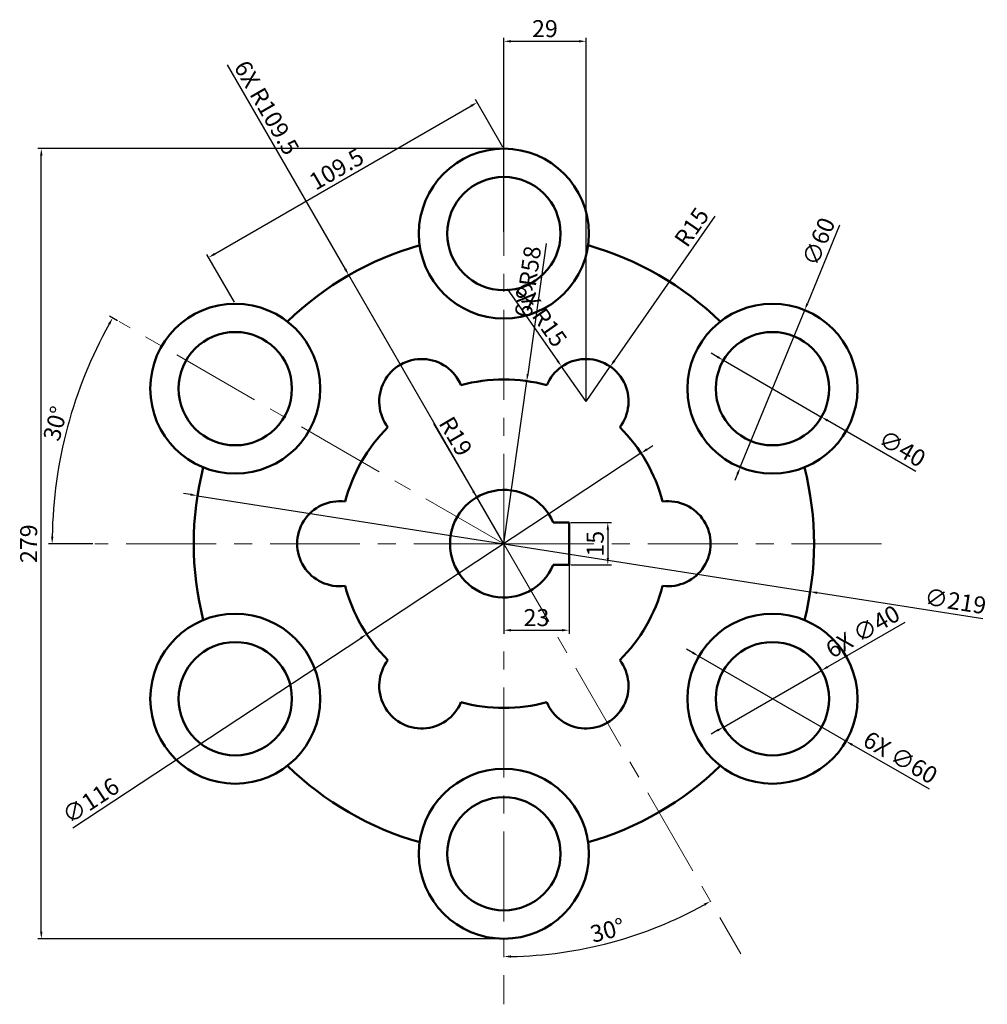
# Model space of a CAD drawing. Units: millimetres. Extents: x 3066 to 3408, y 1460 to 1808.
import ezdxf

# ---------------------------------------------------------------- set-up
doc = ezdxf.new("R2010")
doc.units = ezdxf.units.MM
doc.linetypes.add('CENTER', pattern=[50.8, 31.75, -6.35, 6.35, -6.35])
for name, color, linetype, lineweight in [('M-CNTR', 10, 'CENTER', 18), ('M-DIMS', 120, 'Continuous', 25), ('M-OUTL', 7, 'Continuous', 50)]:
    doc.layers.add(name, color=color, linetype=linetype, lineweight=lineweight)
doc.styles.get("Standard").update_dxf_attribs({"font": 'arial.ttf'})
doc.dimstyles.new('ISO-25', dxfattribs={"dimtxt": 6, "dimasz": 2.5, "dimexe": 1.25, "dimexo": 0.625, "dimtad": 1, "dimtxsty": 'Standard', "dimcen": 2.5, "dimadec": 0, "dimazin": 0, "dimtfac": 1, "dimtmove": 0, "dimatfit": 3, "dimfxl": 1, "dimarcsym": 0})

# ---------------------------------------------------------------- blocks, each defined once
blk = doc.blocks.new('*D1')
at = {"layer": 'Defpoints', "color": 0, "transparency": 16777216}
for p in [(3285.34, 1655.07), (3188.52, 1591.19)]:
    blk.add_point(p, dxfattribs=at)
at = {"layer": 'M-DIMS', "color": 0, "lineweight": -2, "transparency": 16777216}
for p, q in [((3285.34, 1655.07), (3188.52, 1591.19)), ((3287.43, 1656.45), (3289.52, 1657.82)), ((3084.82, 1522.76), (3186.43, 1589.81))]:
    blk.add_line(p, q, dxfattribs=at)
at = {"layer": 'M-DIMS', "color": 0, "transparency": 16777216}
for points in [[(3287.2, 1656.79), (3287.66, 1656.1), (3285.34, 1655.07)], [(3186.21, 1590.16), (3186.66, 1589.46), (3188.52, 1591.19)]]:
    blk.add_solid(points, dxfattribs=at)
at = {"layer": 'M-DIMS', "color": 0, "transparency": 16777216, "insert": (3091.47, 1531.77), "char_height": 6, "attachment_point": 5, "rotation": 33.417}
blk.add_mtext('∅116', dxfattribs=at)
blk = doc.blocks.new('*D2')
at = {"layer": 'Defpoints', "color": 0, "transparency": 16777216}
for p in [(3128.75, 1640.07), (3345.11, 1606.18)]:
    blk.add_point(p, dxfattribs=at)
at = {"layer": 'M-DIMS', "color": 0, "lineweight": -2, "transparency": 16777216}
for p, q in [((3126.28, 1640.46), (3123.81, 1640.85)), ((3128.75, 1640.07), (3345.11, 1606.18)), ((3406.02, 1596.65), (3347.58, 1605.8))]:
    blk.add_line(p, q, dxfattribs=at)
at = {"layer": 'M-DIMS', "color": 0, "transparency": 16777216}
for points in [[(3126.35, 1640.87), (3126.22, 1640.05), (3128.75, 1640.07)], [(3347.65, 1606.21), (3347.52, 1605.39), (3345.11, 1606.18)]]:
    blk.add_solid(points, dxfattribs=at)
at = {"layer": 'M-DIMS', "color": 0, "transparency": 16777216, "insert": (3396.22, 1602.08), "char_height": 6, "attachment_point": 5, "rotation": 351.0986}
blk.add_mtext('∅219', dxfattribs=at)
blk = doc.blocks.new('*D3')
at = {"layer": 'Defpoints', "color": 0, "transparency": 16777216}
for p in [(3314.45, 1687.89), (3349.08, 1667.87)]:
    blk.add_point(p, dxfattribs=at)
at = {"layer": 'M-DIMS', "color": 0, "lineweight": -2, "transparency": 16777216}
for p, q in [((3312.29, 1689.14), (3310.12, 1690.39)), ((3314.45, 1687.89), (3349.08, 1667.87)), ((3382.33, 1648.63), (3351.24, 1666.61))]:
    blk.add_line(p, q, dxfattribs=at)
at = {"layer": 'M-DIMS', "color": 0, "transparency": 16777216}
for points in [[(3312.49, 1689.5), (3312.08, 1688.78), (3314.45, 1687.89)], [(3351.45, 1666.97), (3351.03, 1666.25), (3349.08, 1667.87)]]:
    blk.add_solid(points, dxfattribs=at)
at = {"layer": 'M-DIMS', "color": 0, "transparency": 16777216, "insert": (3377.18, 1656.07), "char_height": 6, "attachment_point": 5, "rotation": 329.9577}
blk.add_mtext('∅40', dxfattribs=at)
blk = doc.blocks.new('*D4')
at = {"layer": 'Defpoints', "color": 0, "transparency": 16777216}
for p in [(3343.14, 1705.64), (3320.38, 1650.12)]:
    blk.add_point(p, dxfattribs=at)
at = {"layer": 'M-DIMS', "color": 0, "lineweight": -2, "transparency": 16777216}
for p, q in [((3355.43, 1735.61), (3344.09, 1707.95)), ((3320.38, 1650.12), (3343.14, 1705.64)), ((3319.44, 1647.81), (3318.49, 1645.49))]:
    blk.add_line(p, q, dxfattribs=at)
at = {"layer": 'M-DIMS', "color": 0, "transparency": 16777216}
for points in [[(3343.71, 1708.11), (3344.48, 1707.79), (3343.14, 1705.64)], [(3319.05, 1647.96), (3319.82, 1647.65), (3320.38, 1650.12)]]:
    blk.add_solid(points, dxfattribs=at)
at = {"layer": 'M-DIMS', "color": 0, "transparency": 16777216, "insert": (3348.76, 1729.51), "char_height": 6, "attachment_point": 5, "rotation": 67.7087}
blk.add_mtext('∅60', dxfattribs=at)
blk = doc.blocks.new('*D5')
at = {"layer": 'Defpoints', "color": 0, "transparency": 16777216}
for p in [(3236.93, 1623.13), (3259.93, 1623.13), (3259.93, 1592.57)]:
    blk.add_point(p, dxfattribs=at)
at = {"layer": 'M-DIMS', "color": 0, "lineweight": -2, "transparency": 16777216}
for p, q in [((3236.93, 1622.5), (3236.93, 1591.32)), ((3259.93, 1622.5), (3259.93, 1591.32)), ((3239.43, 1592.57), (3257.43, 1592.57))]:
    blk.add_line(p, q, dxfattribs=at)
at = {"layer": 'M-DIMS', "color": 0, "transparency": 16777216}
for points in [[(3239.43, 1592.99), (3239.43, 1592.16), (3236.93, 1592.57)], [(3257.43, 1592.99), (3257.43, 1592.16), (3259.93, 1592.57)]]:
    blk.add_solid(points, dxfattribs=at)
at = {"layer": 'M-DIMS', "color": 0, "transparency": 16777216, "insert": (3248.43, 1596.26), "char_height": 6, "attachment_point": 5}
blk.add_mtext('23', dxfattribs=at)
blk = doc.blocks.new('*D6')
at = {"layer": 'Defpoints', "color": 0, "transparency": 16777216}
for p in [(3259.93, 1630.63), (3259.93, 1615.63), (3273.63, 1615.63)]:
    blk.add_point(p, dxfattribs=at)
at = {"layer": 'M-DIMS', "color": 0, "lineweight": -2, "transparency": 16777216}
for p, q in [((3260.56, 1630.63), (3274.88, 1630.63)), ((3273.63, 1628.13), (3273.63, 1618.13)), ((3260.56, 1615.63), (3274.88, 1615.63))]:
    blk.add_line(p, q, dxfattribs=at)
at = {"layer": 'M-DIMS', "color": 0, "transparency": 16777216}
for points in [[(3273.22, 1628.13), (3274.05, 1628.13), (3273.63, 1630.63)], [(3273.22, 1618.13), (3274.05, 1618.13), (3273.63, 1615.63)]]:
    blk.add_solid(points, dxfattribs=at)
at = {"layer": 'M-DIMS', "color": 0, "transparency": 16777216, "insert": (3269.95, 1623.13), "char_height": 6, "attachment_point": 5, "rotation": 90}
blk.add_mtext('15', dxfattribs=at)
blk = doc.blocks.new('*D7')
at = {"layer": 'Defpoints', "color": 0, "transparency": 16777216}
for p in [(3227.34, 1639.53), (3236.93, 1623.13)]:
    blk.add_point(p, dxfattribs=at)
at = {"layer": 'M-DIMS', "color": 0, "lineweight": -2, "transparency": 16777216}
for p, q in [((3212.14, 1665.55), (3226.08, 1641.69)), ((3236.93, 1623.13), (3227.34, 1639.53))]:
    blk.add_line(p, q, dxfattribs=at)
at = {"layer": 'M-DIMS', "color": 0, "transparency": 16777216}
blk.add_solid([(3226.44, 1641.9), (3225.72, 1641.48), (3227.34, 1639.53)], dxfattribs=at)
at = {"layer": 'M-DIMS', "color": 0, "transparency": 16777216, "insert": (3219.26, 1660.67), "char_height": 6, "attachment_point": 5, "rotation": 300.3078}
blk.add_mtext('R19', dxfattribs=at)
blk = doc.blocks.new('*D8')
at = {"layer": 'Defpoints', "color": 0, "transparency": 16777216}
for p in [(3274.49, 1685.68), (3265.93, 1673.36)]:
    blk.add_point(p, dxfattribs=at)
at = {"layer": 'M-DIMS', "color": 0, "lineweight": -2, "transparency": 16777216}
for p, q in [((3311.36, 1738.8), (3275.91, 1687.73)), ((3265.93, 1673.36), (3274.49, 1685.68))]:
    blk.add_line(p, q, dxfattribs=at)
at = {"layer": 'M-DIMS', "color": 0, "transparency": 16777216}
blk.add_solid([(3275.57, 1687.97), (3276.26, 1687.5), (3274.49, 1685.68)], dxfattribs=at)
at = {"layer": 'M-DIMS', "color": 0, "transparency": 16777216, "insert": (3303.88, 1734.48), "char_height": 6, "attachment_point": 5, "rotation": 55.2308}
blk.add_mtext('R15', dxfattribs=at)
blk = doc.blocks.new('*D9')
at = {"layer": 'Defpoints', "color": 0, "transparency": 16777216}
for p in [(3236.93, 1623.13), (3236.93, 1623.13), (3262.25, 1479.55), (3320.53, 1478.33), (3236.93, 1460.48)]:
    blk.add_point(p, dxfattribs=at)
at = {"layer": 'M-DIMS', "color": 0, "lineweight": -2, "transparency": 16777216}
blk.add_arc((3236.93, 1623.13), 145.79, 270.9825, 299.0175, dxfattribs=at)
at = {"layer": 'M-DIMS', "color": 0, "transparency": 16777216}
for points in [[(3307.45, 1496), (3307.86, 1495.28), (3309.83, 1496.87)], [(3239.44, 1476.94), (3239.43, 1477.78), (3236.93, 1477.34)]]:
    blk.add_solid(points, dxfattribs=at)
at = {"layer": 'M-DIMS', "color": 0, "transparency": 16777216, "insert": (3273.71, 1485.87), "char_height": 6, "attachment_point": 5, "rotation": 15}
blk.add_mtext('30°', dxfattribs=at)
blk = doc.blocks.new('*D10')
at = {"layer": 'Defpoints', "color": 0, "transparency": 16777216}
for p in [(3101.08, 1701.56), (3087.08, 1677.67), (3092.48, 1623.13), (3236.93, 1623.13), (3236.93, 1623.13)]:
    blk.add_point(p, dxfattribs=at)
at = {"layer": 'M-DIMS', "color": 0, "lineweight": -2, "transparency": 16777216}
for p, q in [((3100.54, 1701.87), (3097.75, 1703.49)), ((3091.85, 1623.13), (3076.22, 1623.13))]:
    blk.add_line(p, q, dxfattribs=at)
blk.add_arc((3236.93, 1623.13), 159.47, 150.8982, 179.1018, dxfattribs=at)
at = {"layer": 'M-DIMS', "color": 0, "transparency": 16777216}
for points in [[(3097.24, 1700.89), (3097.96, 1700.48), (3098.83, 1702.86)], [(3077.9, 1625.62), (3077.07, 1625.63), (3077.47, 1623.13)]]:
    blk.add_solid(points, dxfattribs=at)
at = {"layer": 'M-DIMS', "color": 0, "transparency": 16777216, "insert": (3079.34, 1665.36), "char_height": 6, "attachment_point": 5, "rotation": 75}
blk.add_mtext('30°', dxfattribs=at)
blk = doc.blocks.new('COUPLING-BOSS-OD60-ID40')
for radius in [30, 20]:
    blk.add_circle((0, 0), radius)
blk = doc.blocks.new('*D12')
at = {"layer": 'Defpoints', "color": 0, "transparency": 16777216}
for p in [(3073.63, 1762.63), (3236.93, 1762.63), (3236.93, 1483.63)]:
    blk.add_point(p, dxfattribs=at)
at = {"layer": 'M-DIMS', "color": 0, "lineweight": -2, "transparency": 16777216}
for p, q in [((3236.31, 1762.63), (3072.38, 1762.63)), ((3073.63, 1486.13), (3073.63, 1760.13)), ((3236.31, 1483.63), (3072.38, 1483.63))]:
    blk.add_line(p, q, dxfattribs=at)
at = {"layer": 'M-DIMS', "color": 0, "transparency": 16777216}
for points in [[(3073.21, 1760.13), (3074.05, 1760.13), (3073.63, 1762.63)], [(3073.21, 1486.13), (3074.05, 1486.13), (3073.63, 1483.63)]]:
    blk.add_solid(points, dxfattribs=at)
at = {"layer": 'M-DIMS', "color": 0, "transparency": 16777216, "insert": (3069.94, 1623.13), "char_height": 6, "attachment_point": 5, "rotation": 90}
blk.add_mtext('279', dxfattribs=at)
blk = doc.blocks.new('*D13')
at = {"layer": 'Defpoints', "color": 0, "transparency": 16777216}
for p in [(3227.51, 1778.95), (3236.93, 1762.63), (3142.1, 1707.88)]:
    blk.add_point(p, dxfattribs=at)
at = {"layer": 'M-DIMS', "color": 0, "lineweight": -2, "transparency": 16777216}
for p, q in [((3134.84, 1725.45), (3225.34, 1777.7)), ((3236.62, 1763.17), (3226.88, 1780.04)), ((3141.79, 1708.42), (3132.05, 1725.29))]:
    blk.add_line(p, q, dxfattribs=at)
at = {"layer": 'M-DIMS', "color": 0, "transparency": 16777216}
for points in [[(3225.13, 1778.06), (3225.55, 1777.34), (3227.51, 1778.95)], [(3134.64, 1725.81), (3135.05, 1725.09), (3132.68, 1724.2)]]:
    blk.add_solid(points, dxfattribs=at)
at = {"layer": 'M-DIMS', "color": 0, "transparency": 16777216, "insert": (3178.25, 1754.77), "char_height": 6, "attachment_point": 5, "rotation": 30}
blk.add_mtext('109.5', dxfattribs=at)
blk = doc.blocks.new('*D14')
at = {"layer": 'Defpoints', "color": 0, "transparency": 16777216}
for p in [(3265.93, 1800.54), (3236.93, 1732.63), (3265.93, 1673.36)]:
    blk.add_point(p, dxfattribs=at)
at = {"layer": 'M-DIMS', "color": 0, "lineweight": -2, "transparency": 16777216}
for p, q in [((3236.93, 1733.25), (3236.93, 1801.79)), ((3265.93, 1673.98), (3265.93, 1801.79)), ((3239.43, 1800.54), (3263.43, 1800.54))]:
    blk.add_line(p, q, dxfattribs=at)
at = {"layer": 'M-DIMS', "color": 0, "transparency": 16777216}
for points in [[(3239.43, 1800.96), (3239.43, 1800.12), (3236.93, 1800.54)], [(3263.43, 1800.96), (3263.43, 1800.12), (3265.93, 1800.54)]]:
    blk.add_solid(points, dxfattribs=at)
at = {"layer": 'M-DIMS', "color": 0, "transparency": 16777216, "insert": (3251.43, 1804.23), "char_height": 6, "attachment_point": 5}
blk.add_mtext('29', dxfattribs=at)
blk = doc.blocks.new('*D15')
at = {"layer": 'Defpoints', "color": 0, "transparency": 16777216}
for p in [(3182.18, 1717.96), (3236.93, 1623.13)]:
    blk.add_point(p, dxfattribs=at)
at = {"layer": 'M-DIMS', "color": 0, "lineweight": -2, "transparency": 16777216}
for p, q in [((3139.28, 1792.27), (3180.93, 1720.12)), ((3236.93, 1623.13), (3182.18, 1717.96))]:
    blk.add_line(p, q, dxfattribs=at)
at = {"layer": 'M-DIMS', "color": 0, "transparency": 16777216}
blk.add_solid([(3181.29, 1720.33), (3180.57, 1719.91), (3182.18, 1717.96)], dxfattribs=at)
at = {"layer": 'M-DIMS', "color": 0, "transparency": 16777216, "insert": (3152.53, 1776.7), "char_height": 6, "attachment_point": 5, "rotation": 300.0001}
blk.add_mtext('6X R109.5', dxfattribs=at)
blk = doc.blocks.new('*D16')
at = {"layer": 'Defpoints', "color": 0, "transparency": 16777216}
for p in [(3245, 1680.56), (3236.93, 1623.13)]:
    blk.add_point(p, dxfattribs=at)
at = {"layer": 'M-DIMS', "color": 0, "lineweight": -2, "transparency": 16777216}
for p, q in [((3251.82, 1729.15), (3245.35, 1683.04)), ((3236.93, 1623.13), (3245, 1680.56))]:
    blk.add_line(p, q, dxfattribs=at)
at = {"layer": 'M-DIMS', "color": 0, "transparency": 16777216}
blk.add_solid([(3244.94, 1683.1), (3245.76, 1682.98), (3245, 1680.56)], dxfattribs=at)
at = {"layer": 'M-DIMS', "color": 0, "transparency": 16777216, "insert": (3246.19, 1715.54), "char_height": 6, "attachment_point": 5, "rotation": 82.0047}
blk.add_mtext('6X R58', dxfattribs=at)
blk = doc.blocks.new('*D17')
at = {"layer": 'Defpoints', "color": 0, "transparency": 16777216}
for p in [(3257.33, 1685.65), (3265.93, 1673.36)]:
    blk.add_point(p, dxfattribs=at)
at = {"layer": 'M-DIMS', "color": 0, "lineweight": -2, "transparency": 16777216}
for p, q in [((3238.09, 1713.14), (3255.9, 1687.69)), ((3265.93, 1673.36), (3257.33, 1685.65))]:
    blk.add_line(p, q, dxfattribs=at)
at = {"layer": 'M-DIMS', "color": 0, "transparency": 16777216}
blk.add_solid([(3256.24, 1687.93), (3255.56, 1687.46), (3257.33, 1685.65)], dxfattribs=at)
at = {"layer": 'M-DIMS', "color": 0, "transparency": 16777216, "insert": (3249.3, 1703.56), "char_height": 6, "attachment_point": 5, "rotation": 304.9873}
blk.add_mtext('6X R15', dxfattribs=at)
blk = doc.blocks.new('*D18')
at = {"layer": 'Defpoints', "color": 0, "transparency": 16777216}
for p in [(3305.78, 1583.38), (3357.74, 1553.38)]:
    blk.add_point(p, dxfattribs=at)
at = {"layer": 'M-DIMS', "color": 0, "lineweight": -2, "transparency": 16777216}
for p, q in [((3303.62, 1584.63), (3301.45, 1585.88)), ((3305.78, 1583.38), (3357.74, 1553.38)), ((3387.15, 1536.4), (3359.91, 1552.13))]:
    blk.add_line(p, q, dxfattribs=at)
at = {"layer": 'M-DIMS', "color": 0, "transparency": 16777216}
for points in [[(3303.83, 1584.99), (3303.41, 1584.27), (3305.78, 1583.38)], [(3360.12, 1552.49), (3359.7, 1551.77), (3357.74, 1553.38)]]:
    blk.add_solid(points, dxfattribs=at)
at = {"layer": 'M-DIMS', "color": 0, "transparency": 16777216, "insert": (3376.54, 1546.98), "char_height": 6, "attachment_point": 5, "rotation": 330.0011}
blk.add_mtext('6X ∅60', dxfattribs=at)
blk = doc.blocks.new('*D19')
at = {"layer": 'Defpoints', "color": 0, "transparency": 16777216}
for p in [(3349.08, 1578.38), (3314.44, 1558.38)]:
    blk.add_point(p, dxfattribs=at)
at = {"layer": 'M-DIMS', "color": 0, "lineweight": -2, "transparency": 16777216}
for p, q in [((3378.49, 1595.36), (3351.25, 1579.63)), ((3314.44, 1558.38), (3349.08, 1578.38)), ((3312.28, 1557.13), (3310.11, 1555.88))]:
    blk.add_line(p, q, dxfattribs=at)
at = {"layer": 'M-DIMS', "color": 0, "transparency": 16777216}
for points in [[(3351.04, 1579.99), (3351.46, 1579.27), (3349.08, 1578.38)], [(3312.07, 1557.49), (3312.49, 1556.77), (3314.44, 1558.38)]]:
    blk.add_solid(points, dxfattribs=at)
at = {"layer": 'M-DIMS', "color": 0, "transparency": 16777216, "insert": (3364.02, 1591.46), "char_height": 6, "attachment_point": 5, "rotation": 30.005}
blk.add_mtext('6X ∅40', dxfattribs=at)

msp = doc.modelspace()

# ---------------------------------------------------------------- linework, layer by layer
at = {"layer": 'M-CNTR'}
for q in [(3236.933, 1781.691), (3101.085, 1701.56), (3092.479, 1623.128), (3236.933, 1460.483), (3375.795, 1623.128), (3320.534, 1478.328)]:
    msp.add_line((3236.933, 1623.128), q, dxfattribs=at)
at = {"layer": 'M-OUTL'}
for p, q in [((3254.39, 1630.628), (3259.933, 1630.628)), ((3259.933, 1630.628), (3259.933, 1615.628)), ((3259.933, 1615.628), (3254.39, 1615.628))]:
    msp.add_line(p, q, dxfattribs=at)
for centre, radius, start, end in [((3236.933, 1623.128), 109.5, 105.74699, 134.25301), ((3236.933, 1623.128), 109.5, 45.74699, 74.25301), ((3207.933, 1673.357), 15, 22.57026, 217.42974), ((3265.933, 1673.357), 15, 322.57026, 157.42974), ((3236.933, 1623.128), 58, 74.85948, 105.14052), ((3236.933, 1623.128), 58, 134.85948, 165.14052), ((3236.933, 1623.128), 58, 14.85948, 45.14052), ((3236.933, 1623.128), 109.5, 165.74699, 194.25301), ((3236.933, 1623.128), 109.5, 345.74699, 14.25301), ((3236.933, 1623.128), 19, 23.24956, 336.75044), ((3178.933, 1623.128), 15, 82.57026, 277.42974), ((3294.933, 1623.128), 15, 262.57026, 97.42974), ((3236.933, 1623.128), 58, 194.85948, 225.14052), ((3236.933, 1623.128), 58, 314.85948, 345.14052), ((3207.933, 1572.899), 15, 142.57026, 337.42974), ((3265.933, 1572.899), 15, 202.57026, 37.42974), ((3236.933, 1623.128), 58, 254.85948, 285.14052), ((3236.933, 1623.128), 109.5, 225.74699, 254.25301), ((3236.933, 1623.128), 109.5, 285.74699, 314.25301)]:
    msp.add_arc(centre, radius, start, end, dxfattribs=at)

# ---------------------------------------------------------------- block references
for p in [(3236.933, 1732.628), (3142.103, 1677.878), (3331.763, 1677.878), (3142.103, 1568.378), (3331.763, 1568.378), (3236.933, 1513.628)]:
    msp.add_blockref('COUPLING-BOSS-OD60-ID40', p, dxfattribs=at)

# ---------------------------------------------------------------- dimensions: what is measured, and where the dimension line sits
at = {"layer": 'M-DIMS'}
for base, p1, p2, override, picture, middle in [((3265.933, 1800.541), (3236.933, 1732.628), (3265.933, 1673.357), {"dimdec": 0, "dimlfac": 1, "dimrnd": 0, "dimzin": 0, "dimdsep": 46, "dimlunit": 2}, '*D14', (3251.433, 1804.229)), ((3259.933, 1592.572), (3236.933, 1623.128), (3259.933, 1623.128), {"dimclrd": 0, "dimclre": 0, "dimclrt": 0}, '*D5', (3248.433, 1596.263))]:
    dim = msp.add_linear_dim(base=base, p1=p1, p2=p2, dimstyle='ISO-25', override=override, dxfattribs=at)
    dim.commit()
    dim.dimension.update_dxf_attribs({"geometry": picture, "text_midpoint": middle})
for mpoint, override, picture, middle in [((3182.183, 1717.958), {"dimdec": 1, "dimlfac": 1, "dimrnd": 0, "dimzin": 0, "dimdsep": 46, "dimlunit": 2}, '*D15', (3149.333, 1774.856)), ((3245.001, 1680.564), {"dimdec": 0, "dimlfac": 1, "dimrnd": 0, "dimzin": 0, "dimdsep": 46, "dimlunit": 2}, '*D16', (3249.841, 1715.026))]:
    dim = msp.add_radius_dim(center=(3236.933, 1623.128), mpoint=mpoint, text='6X <>', dimstyle='ISO-25', override=override, dxfattribs=at)
    dim.commit()
    dim.dimension.update_dxf_attribs({"geometry": picture, "text_midpoint": middle, "dimtype": 164})
for base, p1, p2, angle, override, picture, middle in [((3227.508, 1778.953), (3142.103, 1707.878), (3236.933, 1762.628), 30, {"dimdec": 1, "dimlfac": 1, "dimrnd": 0, "dimzin": 0, "dimdsep": 46, "dimlunit": 2}, '*D13', (3178.249, 1754.772)), ((3073.629, 1762.628), (3236.933, 1483.628), (3236.933, 1762.628), 90, {"dimdec": 0, "dimlfac": 1, "dimrnd": 0, "dimzin": 0, "dimdsep": 46, "dimlunit": 2}, '*D12', (3069.941, 1623.128)), ((3273.634, 1615.628), (3259.933, 1630.628), (3259.933, 1615.628), 90, {"dimclrd": 0, "dimclre": 0, "dimclrt": 0}, '*D6', (3269.946, 1623.128))]:
    dim = msp.add_linear_dim(base=base, p1=p1, p2=p2, angle=angle, dimstyle='ISO-25', override=override, dxfattribs=at)
    dim.commit()
    dim.dimension.update_dxf_attribs({"geometry": picture, "text_midpoint": middle})
for center, mpoint, picture, middle in [((3265.933, 1673.357), (3274.487, 1685.679), '*D8', (3306.905, 1732.376)), ((3236.933, 1623.128), (3227.345, 1639.531), '*D7', (3216.074, 1658.814))]:
    dim = msp.add_radius_dim(center=center, mpoint=mpoint, dimstyle='ISO-25', override={"dimclrd": 0, "dimclre": 0, "dimclrt": 0}, dxfattribs=at)
    dim.commit()
    dim.dimension.update_dxf_attribs({"geometry": picture, "text_midpoint": middle, "dimtype": 164})
for p1, p2, picture, middle in [((3320.384, 1650.12), (3343.142, 1705.636), '*D4', (3352.33, 1728.048)), ((3314.45, 1687.891), (3349.076, 1667.865), '*D3', (3375.25, 1652.728)), ((3285.345, 1655.07), (3188.522, 1591.186), '*D1', (3093.594, 1528.552)), ((3128.752, 1640.071), (3345.114, 1606.185), '*D2', (3395.623, 1598.274))]:
    dim = msp.add_diameter_dim_2p(p1=p1, p2=p2, dimstyle='ISO-25', override={"dimclrd": 0, "dimclre": 0, "dimclrt": 0}, dxfattribs=at)
    dim.commit()
    dim.dimension.update_dxf_attribs({"geometry": picture, "text_midpoint": middle, "dimtype": 163})
dim = msp.add_radius_dim(center=(3265.933, 1673.357), mpoint=(3257.332, 1685.647), text='6X <>', dimstyle='ISO-25', override={"dimdec": 0, "dimlfac": 1, "dimrnd": 0, "dimzin": 0, "dimdsep": 46, "dimlunit": 2}, dxfattribs=at)
dim.commit()
dim.dimension.update_dxf_attribs({"geometry": '*D17', "text_midpoint": (3249.3, 1703.556)})
for base, line1, line2, picture, middle in [((3087.083, 1677.669), ((3236.933, 1623.128), (3092.479, 1623.128)), ((3236.933, 1623.128), (3101.085, 1701.56)), '*D10', (3079.335, 1665.356)), ((3262.249, 1479.555), ((3236.933, 1623.128), (3236.933, 1460.483)), ((3236.933, 1623.128), (3320.534, 1478.328)), '*D9', (3273.711, 1485.872))]:
    dim = msp.add_angular_dim_2l(base=base, line1=line1, line2=line2, dimstyle='ISO-25', override={"dimclrd": 0, "dimclre": 0, "dimclrt": 0}, dxfattribs=at)
    dim.commit()
    dim.dimension.update_dxf_attribs({"geometry": picture, "text_midpoint": middle})
for p1, p2, picture, middle in [((3314.443, 1558.376), (3349.083, 1578.38), '*D19', (3365.951, 1588.121)), ((3305.782, 1583.377), (3357.744, 1553.379), '*D18', (3374.614, 1543.639))]:
    dim = msp.add_diameter_dim_2p(p1=p1, p2=p2, text='6X <>', dimstyle='ISO-25', override={"dimdec": 0, "dimlfac": 1, "dimrnd": 0, "dimzin": 0, "dimdsep": 46, "dimlunit": 2}, dxfattribs=at)
    dim.commit()
    dim.dimension.update_dxf_attribs({"geometry": picture, "text_midpoint": middle})

doc.saveas('drawing.dxf')
